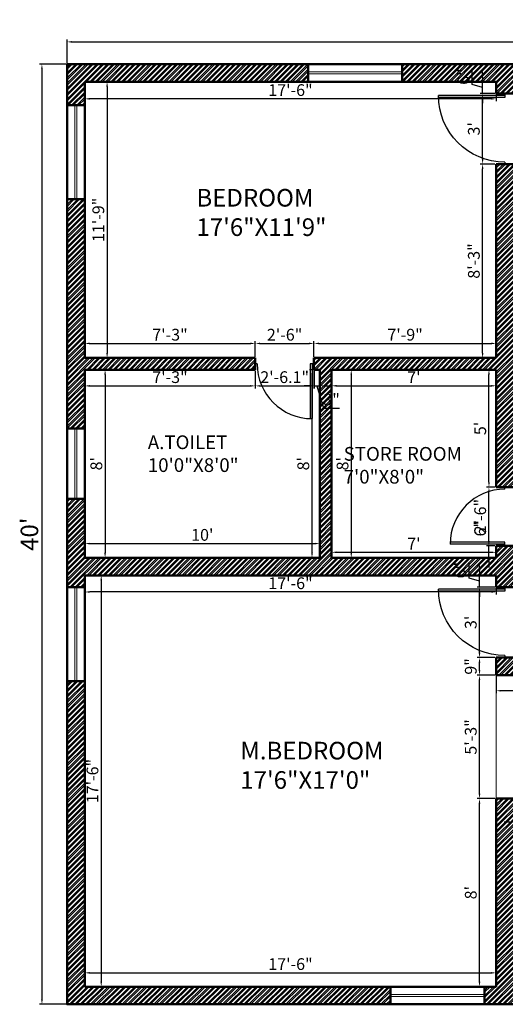
# Model space of a CAD drawing. Units: inches. Extents: x 3590 to 5167, y 65 to 1917.
# Tile 23 of 100: x 4396 to 4644, y 735 to 1238. Entities that reach past the tile are written whole.
import ezdxf

# ---------------------------------------------------------------- set-up
doc = ezdxf.new("R2010")
doc.units = ezdxf.units.IN
doc.linetypes.add('DASHED', pattern=[0.75, 0.5, -0.25])
for name, color, linetype, lineweight in [('A-ANNO-DIMS', 2, 'Continuous', 18), ('A-AREA-IDEN', 7, 'Continuous', 18), ('A-DOOR', 3, 'Continuous', 25), ('A-GLAZ', 4, 'Continuous', 18), ('A-WALL', 7, 'Continuous', 50), ('A-WALL-PATT', 251, 'Continuous', 13), ('S-BEAM-OVHD', 7, 'DASHED', 18)]:
    doc.layers.add(name, color=color, linetype=linetype, lineweight=lineweight)
doc.styles.get("Standard").update_dxf_attribs({"font": 'arial.ttf'})
doc.dimstyles.new('ISO-25', dxfattribs={"dimtxt": 9, "dimasz": 2.5, "dimexe": 1.25, "dimexo": 0.625, "dimtad": 1, "dimdec": 1, "dimlunit": 3, "dimtxsty": 'Standard', "dimcen": 2.5, "dimadec": 0, "dimazin": 0, "dimtfac": 1, "dimtdec": 1, "dimtmove": 0, "dimatfit": 3, "dimfxl": 1, "dimarcsym": 0})

# ---------------------------------------------------------------- blocks, each defined once
blk = doc.blocks.new('*D105')
at = {"layer": 'A-ANNO-DIMS', "color": 0, "lineweight": -2, "transparency": 16777216}
for p, q in [((4420.27, 1215.97), (4420.27, 1227.96)), ((4422.77, 1226.71), (5077.77, 1226.71)), ((5080.27, 1215.97), (5080.27, 1227.96))]:
    blk.add_line(p, q, dxfattribs=at)
at = {"layer": 'A-ANNO-DIMS', "color": 0, "transparency": 16777216}
for points in [[(4422.77, 1227.13), (4422.77, 1226.29), (4420.27, 1226.71)], [(5077.77, 1227.13), (5077.77, 1226.29), (5080.27, 1226.71)]]:
    blk.add_solid(points, dxfattribs=at)
at = {"layer": 'Defpoints', "color": 0, "transparency": 16777216}
for p in [(5080.27, 1226.71), (4420.27, 1215.35), (5080.27, 1215.35)]:
    blk.add_point(p, dxfattribs=at)
at = {"layer": 'A-ANNO-DIMS', "color": 0, "transparency": 16777216, "insert": (4750.27, 1231.91), "char_height": 9, "attachment_point": 5}
blk.add_mtext("55'", dxfattribs=at)
blk = doc.blocks.new('*D106')
at = {"layer": 'A-ANNO-DIMS', "color": 0, "lineweight": -2, "transparency": 16777216}
for p, q in [((4419.65, 1215.35), (4406.15, 1215.35)), ((4407.4, 1212.85), (4407.4, 737.85)), ((4419.65, 735.35), (4406.15, 735.35))]:
    blk.add_line(p, q, dxfattribs=at)
at = {"layer": 'A-ANNO-DIMS', "color": 0, "transparency": 16777216}
for points in [[(4406.98, 1212.85), (4407.82, 1212.85), (4407.4, 1215.35)], [(4406.98, 737.85), (4407.82, 737.85), (4407.4, 735.35)]]:
    blk.add_solid(points, dxfattribs=at)
at = {"layer": 'Defpoints', "color": 0, "transparency": 16777216}
for p in [(4420.27, 1215.35), (4407.4, 735.35), (4420.27, 735.35)]:
    blk.add_point(p, dxfattribs=at)
at = {"layer": 'A-ANNO-DIMS', "color": 0, "transparency": 16777216, "insert": (4402.18, 975.35), "char_height": 9, "attachment_point": 5, "rotation": 90}
blk.add_mtext("40'", dxfattribs=at)
blk = doc.blocks.new('D1')
for p, q in [((1, 0), (1, 34)), ((2, 0), (2, 33.99)), ((0, 0), (2, 0)), ((35, 0), (36, 0))]:
    blk.add_line(p, q)
at = {"ltscale": 0.5}
blk.add_arc((1, 0), 34, 0, 90, dxfattribs=at)
blk = doc.blocks.new('D2')
for p, q in [((1, 0), (1, 28)), ((2, 0), (2, 27.98)), ((0, 0), (2, 0)), ((29, 0), (30, 0))]:
    blk.add_line(p, q)
at = {"ltscale": 0.5}
blk.add_arc((1, 0), 28, 0, 90, dxfattribs=at)
blk = doc.blocks.new('*D107')
at = {"layer": 'A-ANNO-DIMS', "color": 0, "lineweight": -2, "transparency": 16777216}
for p, q in [((4429.27, 1205.72), (4429.27, 1196.39)), ((4639.27, 1205.72), (4639.27, 1196.39)), ((4636.77, 1197.64), (4431.77, 1197.64))]:
    blk.add_line(p, q, dxfattribs=at)
at = {"layer": 'A-ANNO-DIMS', "color": 0, "transparency": 16777216}
for points in [[(4431.77, 1198.06), (4431.77, 1197.22), (4429.27, 1197.64)], [(4636.77, 1198.06), (4636.77, 1197.22), (4639.27, 1197.64)]]:
    blk.add_solid(points, dxfattribs=at)
at = {"layer": 'Defpoints', "color": 0, "transparency": 16777216}
for p in [(4429.27, 1206.35), (4639.27, 1206.35), (4429.27, 1197.64)]:
    blk.add_point(p, dxfattribs=at)
at = {"layer": 'A-ANNO-DIMS', "color": 0, "transparency": 16777216, "insert": (4534.27, 1201.33), "char_height": 6, "attachment_point": 5}
blk.add_mtext('17\'-6"', dxfattribs=at)
blk = doc.blocks.new('*D108')
at = {"layer": 'A-ANNO-DIMS', "color": 0, "lineweight": -2, "transparency": 16777216}
for p, q in [((4429.9, 1206.35), (4441.91, 1206.35)), ((4440.66, 1203.85), (4440.66, 1067.85)), ((4429.9, 1065.35), (4441.91, 1065.35))]:
    blk.add_line(p, q, dxfattribs=at)
at = {"layer": 'A-ANNO-DIMS', "color": 0, "transparency": 16777216}
for points in [[(4440.24, 1203.85), (4441.08, 1203.85), (4440.66, 1206.35)], [(4440.24, 1067.85), (4441.08, 1067.85), (4440.66, 1065.35)]]:
    blk.add_solid(points, dxfattribs=at)
at = {"layer": 'Defpoints', "color": 0, "transparency": 16777216}
for p in [(4429.27, 1206.35), (4429.27, 1065.35), (4440.66, 1065.35)]:
    blk.add_point(p, dxfattribs=at)
at = {"layer": 'A-ANNO-DIMS', "color": 0, "transparency": 16777216, "insert": (4436.97, 1135.85), "char_height": 6, "attachment_point": 5, "rotation": 90}
blk.add_mtext('11\'-9"', dxfattribs=at)
blk = doc.blocks.new('*D109')
at = {"layer": 'A-ANNO-DIMS', "color": 0, "lineweight": -2, "transparency": 16777216}
for p, q in [((4429.27, 1065.97), (4429.27, 1074)), ((4431.77, 1072.75), (4513.77, 1072.75)), ((4516.27, 1065.97), (4516.27, 1074))]:
    blk.add_line(p, q, dxfattribs=at)
at = {"layer": 'A-ANNO-DIMS', "color": 0, "transparency": 16777216}
for points in [[(4431.77, 1073.17), (4431.77, 1072.33), (4429.27, 1072.75)], [(4513.77, 1073.17), (4513.77, 1072.33), (4516.27, 1072.75)]]:
    blk.add_solid(points, dxfattribs=at)
at = {"layer": 'Defpoints', "color": 0, "transparency": 16777216}
for p in [(4516.27, 1072.75), (4429.27, 1065.35), (4516.27, 1065.35)]:
    blk.add_point(p, dxfattribs=at)
at = {"layer": 'A-ANNO-DIMS', "color": 0, "transparency": 16777216, "insert": (4472.77, 1076.44), "char_height": 6, "attachment_point": 5}
blk.add_mtext('7\'-3"', dxfattribs=at)
blk = doc.blocks.new('*D110')
at = {"layer": 'A-ANNO-DIMS', "color": 0, "lineweight": -2, "transparency": 16777216}
for p, q in [((4516.27, 1065.97), (4516.27, 1074)), ((4518.77, 1072.75), (4543.77, 1072.75)), ((4546.27, 1065.97), (4546.27, 1074))]:
    blk.add_line(p, q, dxfattribs=at)
at = {"layer": 'A-ANNO-DIMS', "color": 0, "transparency": 16777216}
for points in [[(4518.77, 1073.17), (4518.77, 1072.33), (4516.27, 1072.75)], [(4543.77, 1073.17), (4543.77, 1072.33), (4546.27, 1072.75)]]:
    blk.add_solid(points, dxfattribs=at)
at = {"layer": 'Defpoints', "color": 0, "transparency": 16777216}
for p in [(4546.27, 1072.75), (4516.27, 1065.35), (4546.27, 1065.35)]:
    blk.add_point(p, dxfattribs=at)
at = {"layer": 'A-ANNO-DIMS', "color": 0, "transparency": 16777216, "insert": (4531.27, 1076.44), "char_height": 6, "attachment_point": 5}
blk.add_mtext('2\'-6"', dxfattribs=at)
blk = doc.blocks.new('*D111')
at = {"layer": 'A-ANNO-DIMS', "color": 0, "lineweight": -2, "transparency": 16777216}
for p, q in [((4546.27, 1065.97), (4546.27, 1074)), ((4548.77, 1072.75), (4636.77, 1072.75)), ((4639.27, 1065.97), (4639.27, 1074))]:
    blk.add_line(p, q, dxfattribs=at)
at = {"layer": 'A-ANNO-DIMS', "color": 0, "transparency": 16777216}
for points in [[(4548.77, 1073.17), (4548.77, 1072.33), (4546.27, 1072.75)], [(4636.77, 1073.17), (4636.77, 1072.33), (4639.27, 1072.75)]]:
    blk.add_solid(points, dxfattribs=at)
at = {"layer": 'Defpoints', "color": 0, "transparency": 16777216}
for p in [(4639.27, 1072.75), (4546.27, 1065.35), (4639.27, 1065.35)]:
    blk.add_point(p, dxfattribs=at)
at = {"layer": 'A-ANNO-DIMS', "color": 0, "transparency": 16777216, "insert": (4592.77, 1076.44), "char_height": 6, "attachment_point": 5}
blk.add_mtext('7\'-9"', dxfattribs=at)
blk = doc.blocks.new('*D112')
at = {"layer": 'A-ANNO-DIMS', "color": 0, "lineweight": -2, "transparency": 16777216}
for p, q in [((4638.65, 1164.35), (4631.09, 1164.35)), ((4632.34, 1067.85), (4632.34, 1161.85)), ((4638.65, 1065.35), (4631.09, 1065.35))]:
    blk.add_line(p, q, dxfattribs=at)
at = {"layer": 'A-ANNO-DIMS', "color": 0, "transparency": 16777216}
for points in [[(4631.93, 1161.85), (4632.76, 1161.85), (4632.34, 1164.35)], [(4631.93, 1067.85), (4632.76, 1067.85), (4632.34, 1065.35)]]:
    blk.add_solid(points, dxfattribs=at)
at = {"layer": 'Defpoints', "color": 0, "transparency": 16777216}
for p in [(4632.34, 1164.35), (4639.27, 1164.35), (4639.27, 1065.35)]:
    blk.add_point(p, dxfattribs=at)
at = {"layer": 'A-ANNO-DIMS', "color": 0, "transparency": 16777216, "insert": (4628.65, 1114.85), "char_height": 6, "attachment_point": 5, "rotation": 90}
blk.add_mtext('8\'-3"', dxfattribs=at)
blk = doc.blocks.new('*D113')
at = {"layer": 'A-ANNO-DIMS', "color": 0, "lineweight": -2, "transparency": 16777216}
for p, q in [((4638.65, 1200.35), (4631.09, 1200.35)), ((4632.34, 1166.85), (4632.34, 1197.85)), ((4638.65, 1164.35), (4631.09, 1164.35))]:
    blk.add_line(p, q, dxfattribs=at)
at = {"layer": 'A-ANNO-DIMS', "color": 0, "transparency": 16777216}
for points in [[(4631.93, 1197.85), (4632.76, 1197.85), (4632.34, 1200.35)], [(4631.93, 1166.85), (4632.76, 1166.85), (4632.34, 1164.35)]]:
    blk.add_solid(points, dxfattribs=at)
at = {"layer": 'Defpoints', "color": 0, "transparency": 16777216}
for p in [(4632.34, 1200.35), (4639.27, 1200.35), (4639.27, 1164.35)]:
    blk.add_point(p, dxfattribs=at)
at = {"layer": 'A-ANNO-DIMS', "color": 0, "transparency": 16777216, "insert": (4628.65, 1182.35), "char_height": 6, "attachment_point": 5, "rotation": 90}
blk.add_mtext("3'", dxfattribs=at)
blk = doc.blocks.new('*D114')
at = {"layer": 'A-ANNO-DIMS', "color": 0, "lineweight": -2, "transparency": 16777216}
for p, q in [((4627.09, 1204.92), (4627.09, 1213.1)), ((4632.34, 1208.85), (4632.34, 1211.35)), ((4632.34, 1203.35), (4627.09, 1204.92)), ((4638.65, 1206.35), (4631.09, 1206.35)), ((4632.34, 1200.35), (4632.34, 1206.35)), ((4632.34, 1200.35), (4632.34, 1206.35)), ((4638.65, 1200.35), (4631.09, 1200.35)), ((4632.34, 1197.85), (4632.34, 1195.35))]:
    blk.add_line(p, q, dxfattribs=at)
at = {"layer": 'A-ANNO-DIMS', "color": 0, "transparency": 16777216}
for points in [[(4631.93, 1208.85), (4632.76, 1208.85), (4632.34, 1206.35)], [(4631.93, 1197.85), (4632.76, 1197.85), (4632.34, 1200.35)]]:
    blk.add_solid(points, dxfattribs=at)
at = {"layer": 'Defpoints', "color": 0, "transparency": 16777216}
for p in [(4632.34, 1206.35), (4639.27, 1206.35), (4639.27, 1200.35)]:
    blk.add_point(p, dxfattribs=at)
at = {"layer": 'A-ANNO-DIMS', "color": 0, "transparency": 16777216, "insert": (4623.4, 1209.01), "char_height": 6, "attachment_point": 5, "rotation": 90}
blk.add_mtext('6"', dxfattribs=at)
blk = doc.blocks.new('*D115')
at = {"layer": 'A-ANNO-DIMS', "color": 0, "lineweight": -2, "transparency": 16777216}
for p, q in [((4429.9, 1059.35), (4440.89, 1059.35)), ((4439.64, 1056.85), (4439.64, 965.85)), ((4429.9, 963.35), (4440.89, 963.35))]:
    blk.add_line(p, q, dxfattribs=at)
at = {"layer": 'A-ANNO-DIMS', "color": 0, "transparency": 16777216}
for points in [[(4439.22, 1056.85), (4440.05, 1056.85), (4439.64, 1059.35)], [(4439.22, 965.85), (4440.05, 965.85), (4439.64, 963.35)]]:
    blk.add_solid(points, dxfattribs=at)
at = {"layer": 'Defpoints', "color": 0, "transparency": 16777216}
for p in [(4429.27, 1059.35), (4429.27, 963.35), (4439.64, 963.35)]:
    blk.add_point(p, dxfattribs=at)
at = {"layer": 'A-ANNO-DIMS', "color": 0, "transparency": 16777216, "insert": (4435.95, 1011.35), "char_height": 6, "attachment_point": 5, "rotation": 90}
blk.add_mtext("8'", dxfattribs=at)
blk = doc.blocks.new('*D116')
at = {"layer": 'A-ANNO-DIMS', "color": 0, "lineweight": -2, "transparency": 16777216}
for p, q in [((4429.27, 963.97), (4429.27, 971.82)), ((4431.77, 970.57), (4546.77, 970.57)), ((4549.27, 963.97), (4549.27, 971.82))]:
    blk.add_line(p, q, dxfattribs=at)
at = {"layer": 'A-ANNO-DIMS', "color": 0, "transparency": 16777216}
for points in [[(4431.77, 970.98), (4431.77, 970.15), (4429.27, 970.57)], [(4546.77, 970.98), (4546.77, 970.15), (4549.27, 970.57)]]:
    blk.add_solid(points, dxfattribs=at)
at = {"layer": 'Defpoints', "color": 0, "transparency": 16777216}
for p in [(4549.27, 970.57), (4429.27, 963.35), (4549.27, 963.35)]:
    blk.add_point(p, dxfattribs=at)
at = {"layer": 'A-ANNO-DIMS', "color": 0, "transparency": 16777216, "insert": (4489.27, 974.25), "char_height": 6, "attachment_point": 5}
blk.add_mtext("10'", dxfattribs=at)
blk = doc.blocks.new('*D117')
at = {"layer": 'A-ANNO-DIMS', "color": 0, "lineweight": -2, "transparency": 16777216}
for p, q in [((4548.65, 1059.35), (4544.02, 1059.35)), ((4545.27, 965.85), (4545.27, 1056.85)), ((4548.65, 963.35), (4544.02, 963.35))]:
    blk.add_line(p, q, dxfattribs=at)
at = {"layer": 'A-ANNO-DIMS', "color": 0, "transparency": 16777216}
for points in [[(4544.86, 1056.85), (4545.69, 1056.85), (4545.27, 1059.35)], [(4544.86, 965.85), (4545.69, 965.85), (4545.27, 963.35)]]:
    blk.add_solid(points, dxfattribs=at)
at = {"layer": 'Defpoints', "color": 0, "transparency": 16777216}
for p in [(4545.27, 1059.35), (4549.27, 1059.35), (4549.27, 963.35)]:
    blk.add_point(p, dxfattribs=at)
at = {"layer": 'A-ANNO-DIMS', "color": 0, "transparency": 16777216, "insert": (4541.59, 1011.35), "char_height": 6, "attachment_point": 5, "rotation": 90}
blk.add_mtext("8'", dxfattribs=at)
blk = doc.blocks.new('*D118')
at = {"layer": 'A-ANNO-DIMS', "color": 0, "lineweight": -2, "transparency": 16777216}
for p, q in [((4429.27, 1058.72), (4429.27, 1049.83)), ((4516.27, 1058.72), (4516.27, 1049.83)), ((4431.77, 1051.08), (4513.77, 1051.08))]:
    blk.add_line(p, q, dxfattribs=at)
at = {"layer": 'A-ANNO-DIMS', "color": 0, "transparency": 16777216}
for points in [[(4431.77, 1051.5), (4431.77, 1050.67), (4429.27, 1051.08)], [(4513.77, 1051.5), (4513.77, 1050.67), (4516.27, 1051.08)]]:
    blk.add_solid(points, dxfattribs=at)
at = {"layer": 'Defpoints', "color": 0, "transparency": 16777216}
for p in [(4429.27, 1059.35), (4516.27, 1059.35), (4516.27, 1051.08)]:
    blk.add_point(p, dxfattribs=at)
at = {"layer": 'A-ANNO-DIMS', "color": 0, "transparency": 16777216, "insert": (4472.77, 1054.77), "char_height": 6, "attachment_point": 5}
blk.add_mtext('7\'-3"', dxfattribs=at)
blk = doc.blocks.new('*D119')
at = {"layer": 'A-ANNO-DIMS', "color": 0, "lineweight": -2, "transparency": 16777216}
for p, q in [((4516.27, 1058.72), (4516.27, 1049.83)), ((4546.34, 1058.72), (4546.34, 1049.83)), ((4518.77, 1051.08), (4543.84, 1051.08))]:
    blk.add_line(p, q, dxfattribs=at)
at = {"layer": 'A-ANNO-DIMS', "color": 0, "transparency": 16777216}
for points in [[(4518.77, 1051.5), (4518.77, 1050.67), (4516.27, 1051.08)], [(4543.84, 1051.5), (4543.84, 1050.67), (4546.34, 1051.08)]]:
    blk.add_solid(points, dxfattribs=at)
at = {"layer": 'Defpoints', "color": 0, "transparency": 16777216}
for p in [(4516.27, 1059.35), (4546.34, 1059.35), (4546.34, 1051.08)]:
    blk.add_point(p, dxfattribs=at)
at = {"layer": 'A-ANNO-DIMS', "color": 0, "transparency": 16777216, "insert": (4531.31, 1054.77), "char_height": 6, "attachment_point": 5}
blk.add_mtext('2\'-6.1"', dxfattribs=at)
blk = doc.blocks.new('*D120')
at = {"layer": 'A-ANNO-DIMS', "color": 0, "lineweight": -2, "transparency": 16777216}
for p, q in [((4546.27, 1058.72), (4546.27, 1049.83)), ((4549.27, 1058.72), (4549.27, 1049.83)), ((4543.77, 1051.08), (4541.27, 1051.08)), ((4546.27, 1051.08), (4549.27, 1051.08)), ((4546.27, 1051.08), (4549.27, 1051.08)), ((4547.77, 1051.08), (4551.19, 1039.7)), ((4551.77, 1051.08), (4554.27, 1051.08)), ((4551.19, 1039.7), (4559.33, 1039.7))]:
    blk.add_line(p, q, dxfattribs=at)
at = {"layer": 'A-ANNO-DIMS', "color": 0, "transparency": 16777216}
for points in [[(4543.77, 1051.5), (4543.77, 1050.67), (4546.27, 1051.08)], [(4551.77, 1051.5), (4551.77, 1050.67), (4549.27, 1051.08)]]:
    blk.add_solid(points, dxfattribs=at)
at = {"layer": 'Defpoints', "color": 0, "transparency": 16777216}
for p in [(4546.27, 1059.35), (4549.27, 1059.35), (4549.27, 1051.08)]:
    blk.add_point(p, dxfattribs=at)
at = {"layer": 'A-ANNO-DIMS', "color": 0, "transparency": 16777216, "insert": (4555.26, 1043.39), "char_height": 6, "attachment_point": 5}
blk.add_mtext('3"', dxfattribs=at)
blk = doc.blocks.new('*D121')
at = {"layer": 'A-ANNO-DIMS', "color": 0, "lineweight": -2, "transparency": 16777216}
for p, q in [((4555.27, 1058.72), (4555.27, 1049.87)), ((4639.27, 1058.72), (4639.27, 1049.87)), ((4557.77, 1051.12), (4636.77, 1051.12))]:
    blk.add_line(p, q, dxfattribs=at)
at = {"layer": 'A-ANNO-DIMS', "color": 0, "transparency": 16777216}
for points in [[(4557.77, 1051.54), (4557.77, 1050.71), (4555.27, 1051.12)], [(4636.77, 1051.54), (4636.77, 1050.71), (4639.27, 1051.12)]]:
    blk.add_solid(points, dxfattribs=at)
at = {"layer": 'Defpoints', "color": 0, "transparency": 16777216}
for p in [(4555.27, 1059.35), (4639.27, 1059.35), (4639.27, 1051.12)]:
    blk.add_point(p, dxfattribs=at)
at = {"layer": 'A-ANNO-DIMS', "color": 0, "transparency": 16777216, "insert": (4597.27, 1054.75), "char_height": 6, "attachment_point": 5}
blk.add_mtext("7'", dxfattribs=at)
blk = doc.blocks.new('*D122')
at = {"layer": 'A-ANNO-DIMS', "color": 0, "lineweight": -2, "transparency": 16777216}
for p, q in [((4555.9, 1059.35), (4566.54, 1059.35)), ((4565.29, 1056.85), (4565.29, 965.85)), ((4555.9, 963.35), (4566.54, 963.35))]:
    blk.add_line(p, q, dxfattribs=at)
at = {"layer": 'A-ANNO-DIMS', "color": 0, "transparency": 16777216}
for points in [[(4564.88, 1056.85), (4565.71, 1056.85), (4565.29, 1059.35)], [(4564.88, 965.85), (4565.71, 965.85), (4565.29, 963.35)]]:
    blk.add_solid(points, dxfattribs=at)
at = {"layer": 'Defpoints', "color": 0, "transparency": 16777216}
for p in [(4555.27, 1059.35), (4555.27, 963.35), (4565.29, 963.35)]:
    blk.add_point(p, dxfattribs=at)
at = {"layer": 'A-ANNO-DIMS', "color": 0, "transparency": 16777216, "insert": (4561.61, 1011.35), "char_height": 6, "attachment_point": 5, "rotation": 90}
blk.add_mtext("8'", dxfattribs=at)
blk = doc.blocks.new('*D123')
at = {"layer": 'A-ANNO-DIMS', "color": 0, "lineweight": -2, "transparency": 16777216}
for p, q in [((4555.27, 963.97), (4555.27, 967.37)), ((4557.77, 966.12), (4636.77, 966.12)), ((4639.27, 963.97), (4639.27, 967.37))]:
    blk.add_line(p, q, dxfattribs=at)
at = {"layer": 'A-ANNO-DIMS', "color": 0, "transparency": 16777216}
for points in [[(4557.77, 966.54), (4557.77, 965.71), (4555.27, 966.12)], [(4636.77, 966.54), (4636.77, 965.71), (4639.27, 966.12)]]:
    blk.add_solid(points, dxfattribs=at)
at = {"layer": 'Defpoints', "color": 0, "transparency": 16777216}
for p in [(4639.27, 966.12), (4555.27, 963.35), (4639.27, 963.35)]:
    blk.add_point(p, dxfattribs=at)
at = {"layer": 'A-ANNO-DIMS', "color": 0, "transparency": 16777216, "insert": (4597.27, 969.75), "char_height": 6, "attachment_point": 5}
blk.add_mtext("7'", dxfattribs=at)
blk = doc.blocks.new('*D124')
at = {"layer": 'A-ANNO-DIMS', "color": 0, "lineweight": -2, "transparency": 16777216}
for p, q in [((4635.58, 971.85), (4635.58, 982.52)), ((4638.65, 969.35), (4634.33, 969.35)), ((4635.58, 963.35), (4635.58, 969.35)), ((4638.65, 963.35), (4634.33, 963.35)), ((4635.58, 960.85), (4635.58, 958.35))]:
    blk.add_line(p, q, dxfattribs=at)
at = {"layer": 'A-ANNO-DIMS', "color": 0, "transparency": 16777216}
for points in [[(4635.17, 971.85), (4636, 971.85), (4635.58, 969.35)], [(4635.17, 960.85), (4636, 960.85), (4635.58, 963.35)]]:
    blk.add_solid(points, dxfattribs=at)
at = {"layer": 'Defpoints', "color": 0, "transparency": 16777216}
for p in [(4635.58, 969.35), (4639.27, 969.35), (4639.27, 963.35)]:
    blk.add_point(p, dxfattribs=at)
at = {"layer": 'A-ANNO-DIMS', "color": 0, "transparency": 16777216, "insert": (4631.89, 978.43), "char_height": 6, "attachment_point": 5, "rotation": 90}
blk.add_mtext('6"', dxfattribs=at)
blk = doc.blocks.new('*D125')
at = {"layer": 'A-ANNO-DIMS', "color": 0, "lineweight": -2, "transparency": 16777216}
for p, q in [((4638.65, 999.35), (4634.33, 999.35)), ((4635.58, 971.85), (4635.58, 996.85)), ((4638.65, 969.35), (4634.33, 969.35))]:
    blk.add_line(p, q, dxfattribs=at)
at = {"layer": 'A-ANNO-DIMS', "color": 0, "transparency": 16777216}
for points in [[(4635.17, 996.85), (4636, 996.85), (4635.58, 999.35)], [(4635.17, 971.85), (4636, 971.85), (4635.58, 969.35)]]:
    blk.add_solid(points, dxfattribs=at)
at = {"layer": 'Defpoints', "color": 0, "transparency": 16777216}
for p in [(4635.58, 999.35), (4639.27, 999.35), (4639.27, 969.35)]:
    blk.add_point(p, dxfattribs=at)
at = {"layer": 'A-ANNO-DIMS', "color": 0, "transparency": 16777216, "insert": (4631.89, 984.35), "char_height": 6, "attachment_point": 5, "rotation": 90}
blk.add_mtext('2\'-6"', dxfattribs=at)
blk = doc.blocks.new('*D126')
at = {"layer": 'A-ANNO-DIMS', "color": 0, "lineweight": -2, "transparency": 16777216}
for p, q in [((4638.65, 1059.35), (4634.33, 1059.35)), ((4635.58, 1001.85), (4635.58, 1056.85)), ((4638.65, 999.35), (4634.33, 999.35))]:
    blk.add_line(p, q, dxfattribs=at)
at = {"layer": 'A-ANNO-DIMS', "color": 0, "transparency": 16777216}
for points in [[(4635.17, 1056.85), (4636, 1056.85), (4635.58, 1059.35)], [(4635.17, 1001.85), (4636, 1001.85), (4635.58, 999.35)]]:
    blk.add_solid(points, dxfattribs=at)
at = {"layer": 'Defpoints', "color": 0, "transparency": 16777216}
for p in [(4635.58, 1059.35), (4639.27, 1059.35), (4639.27, 999.35)]:
    blk.add_point(p, dxfattribs=at)
at = {"layer": 'A-ANNO-DIMS', "color": 0, "transparency": 16777216, "insert": (4631.91, 1029.35), "char_height": 6, "attachment_point": 5, "rotation": 90}
blk.add_mtext("5'", dxfattribs=at)
blk = doc.blocks.new('*D127')
at = {"layer": 'A-ANNO-DIMS', "color": 0, "lineweight": -2, "transparency": 16777216}
for p, q in [((4429.27, 953.72), (4429.27, 944.61)), ((4639.27, 953.72), (4639.27, 944.61)), ((4636.77, 945.86), (4431.77, 945.86))]:
    blk.add_line(p, q, dxfattribs=at)
at = {"layer": 'A-ANNO-DIMS', "color": 0, "transparency": 16777216}
for points in [[(4431.77, 946.28), (4431.77, 945.44), (4429.27, 945.86)], [(4636.77, 946.28), (4636.77, 945.44), (4639.27, 945.86)]]:
    blk.add_solid(points, dxfattribs=at)
at = {"layer": 'Defpoints', "color": 0, "transparency": 16777216}
for p in [(4429.27, 954.35), (4639.27, 954.35), (4429.27, 945.86)]:
    blk.add_point(p, dxfattribs=at)
at = {"layer": 'A-ANNO-DIMS', "color": 0, "transparency": 16777216, "insert": (4534.27, 949.55), "char_height": 6, "attachment_point": 5}
blk.add_mtext('17\'-6"', dxfattribs=at)
blk = doc.blocks.new('*D128')
at = {"layer": 'A-ANNO-DIMS', "color": 0, "lineweight": -2, "transparency": 16777216}
for p, q in [((4429.9, 954.35), (4438.92, 954.35)), ((4437.67, 951.85), (4437.67, 746.85)), ((4429.9, 744.35), (4438.92, 744.35))]:
    blk.add_line(p, q, dxfattribs=at)
at = {"layer": 'A-ANNO-DIMS', "color": 0, "transparency": 16777216}
for points in [[(4437.25, 951.85), (4438.08, 951.85), (4437.67, 954.35)], [(4437.25, 746.85), (4438.08, 746.85), (4437.67, 744.35)]]:
    blk.add_solid(points, dxfattribs=at)
at = {"layer": 'Defpoints', "color": 0, "transparency": 16777216}
for p in [(4429.27, 954.35), (4429.27, 744.35), (4437.67, 744.35)]:
    blk.add_point(p, dxfattribs=at)
at = {"layer": 'A-ANNO-DIMS', "color": 0, "transparency": 16777216, "insert": (4433.98, 849.35), "char_height": 6, "attachment_point": 5, "rotation": 90}
blk.add_mtext('17\'-6"', dxfattribs=at)
blk = doc.blocks.new('*D129')
at = {"layer": 'A-ANNO-DIMS', "color": 0, "lineweight": -2, "transparency": 16777216}
for p, q in [((4429.27, 744.97), (4429.27, 752.66)), ((4431.77, 751.41), (4636.77, 751.41)), ((4639.27, 744.97), (4639.27, 752.66))]:
    blk.add_line(p, q, dxfattribs=at)
at = {"layer": 'A-ANNO-DIMS', "color": 0, "transparency": 16777216}
for points in [[(4431.77, 751.83), (4431.77, 751), (4429.27, 751.41)], [(4636.77, 751.83), (4636.77, 751), (4639.27, 751.41)]]:
    blk.add_solid(points, dxfattribs=at)
at = {"layer": 'Defpoints', "color": 0, "transparency": 16777216}
for p in [(4639.27, 751.41), (4429.27, 744.35), (4639.27, 744.35)]:
    blk.add_point(p, dxfattribs=at)
at = {"layer": 'A-ANNO-DIMS', "color": 0, "transparency": 16777216, "insert": (4534.27, 755.1), "char_height": 6, "attachment_point": 5}
blk.add_mtext('17\'-6"', dxfattribs=at)
blk = doc.blocks.new('*D130')
at = {"layer": 'A-ANNO-DIMS', "color": 0, "lineweight": -2, "transparency": 16777216}
for p, q in [((4638.65, 840.35), (4629.51, 840.35)), ((4630.76, 746.85), (4630.76, 837.85)), ((4638.65, 744.35), (4629.51, 744.35))]:
    blk.add_line(p, q, dxfattribs=at)
at = {"layer": 'A-ANNO-DIMS', "color": 0, "transparency": 16777216}
for points in [[(4630.35, 837.85), (4631.18, 837.85), (4630.76, 840.35)], [(4630.35, 746.85), (4631.18, 746.85), (4630.76, 744.35)]]:
    blk.add_solid(points, dxfattribs=at)
at = {"layer": 'Defpoints', "color": 0, "transparency": 16777216}
for p in [(4630.76, 840.35), (4639.27, 840.35), (4639.27, 744.35)]:
    blk.add_point(p, dxfattribs=at)
at = {"layer": 'A-ANNO-DIMS', "color": 0, "transparency": 16777216, "insert": (4627.08, 792.35), "char_height": 6, "attachment_point": 5, "rotation": 90}
blk.add_mtext("8'", dxfattribs=at)
blk = doc.blocks.new('*D131')
at = {"layer": 'A-ANNO-DIMS', "color": 0, "lineweight": -2, "transparency": 16777216}
for p, q in [((4638.65, 903.35), (4629.51, 903.35)), ((4630.76, 842.85), (4630.76, 900.85)), ((4638.65, 840.35), (4629.51, 840.35))]:
    blk.add_line(p, q, dxfattribs=at)
at = {"layer": 'A-ANNO-DIMS', "color": 0, "transparency": 16777216}
for points in [[(4630.35, 900.85), (4631.18, 900.85), (4630.76, 903.35)], [(4630.35, 842.85), (4631.18, 842.85), (4630.76, 840.35)]]:
    blk.add_solid(points, dxfattribs=at)
at = {"layer": 'Defpoints', "color": 0, "transparency": 16777216}
for p in [(4630.76, 903.35), (4639.27, 903.35), (4639.27, 840.35)]:
    blk.add_point(p, dxfattribs=at)
at = {"layer": 'A-ANNO-DIMS', "color": 0, "transparency": 16777216, "insert": (4627.07, 871.85), "char_height": 6, "attachment_point": 5, "rotation": 90}
blk.add_mtext('5\'-3"', dxfattribs=at)
blk = doc.blocks.new('*D132')
at = {"layer": 'A-ANNO-DIMS', "color": 0, "lineweight": -2, "transparency": 16777216}
for p, q in [((4638.65, 912.35), (4629.51, 912.35)), ((4630.76, 905.85), (4630.76, 909.85)), ((4638.65, 903.35), (4629.51, 903.35))]:
    blk.add_line(p, q, dxfattribs=at)
at = {"layer": 'A-ANNO-DIMS', "color": 0, "transparency": 16777216}
for points in [[(4630.35, 909.85), (4631.18, 909.85), (4630.76, 912.35)], [(4630.35, 905.85), (4631.18, 905.85), (4630.76, 903.35)]]:
    blk.add_solid(points, dxfattribs=at)
at = {"layer": 'Defpoints', "color": 0, "transparency": 16777216}
for p in [(4630.76, 912.35), (4639.27, 912.35), (4639.27, 903.35)]:
    blk.add_point(p, dxfattribs=at)
at = {"layer": 'A-ANNO-DIMS', "color": 0, "transparency": 16777216, "insert": (4627.08, 907.85), "char_height": 6, "attachment_point": 5, "rotation": 90}
blk.add_mtext('9"', dxfattribs=at)
blk = doc.blocks.new('*D133')
at = {"layer": 'A-ANNO-DIMS', "color": 0, "lineweight": -2, "transparency": 16777216}
for p, q in [((4638.65, 948.35), (4629.51, 948.35)), ((4630.76, 914.85), (4630.76, 945.85)), ((4638.65, 912.35), (4629.51, 912.35))]:
    blk.add_line(p, q, dxfattribs=at)
at = {"layer": 'A-ANNO-DIMS', "color": 0, "transparency": 16777216}
for points in [[(4630.35, 945.85), (4631.18, 945.85), (4630.76, 948.35)], [(4630.35, 914.85), (4631.18, 914.85), (4630.76, 912.35)]]:
    blk.add_solid(points, dxfattribs=at)
at = {"layer": 'Defpoints', "color": 0, "transparency": 16777216}
for p in [(4630.76, 948.35), (4639.27, 948.35), (4639.27, 912.35)]:
    blk.add_point(p, dxfattribs=at)
at = {"layer": 'A-ANNO-DIMS', "color": 0, "transparency": 16777216, "insert": (4627.07, 930.35), "char_height": 6, "attachment_point": 5, "rotation": 90}
blk.add_mtext("3'", dxfattribs=at)
blk = doc.blocks.new('*D134')
at = {"layer": 'A-ANNO-DIMS', "color": 0, "lineweight": -2, "transparency": 16777216}
for p, q in [((4625.51, 952.92), (4625.51, 961.1)), ((4630.76, 956.85), (4630.76, 959.35)), ((4630.76, 951.35), (4625.51, 952.92)), ((4638.65, 954.35), (4629.51, 954.35)), ((4630.76, 948.35), (4630.76, 954.35)), ((4630.76, 948.35), (4630.76, 954.35)), ((4638.65, 948.35), (4629.51, 948.35)), ((4630.76, 945.85), (4630.76, 943.35))]:
    blk.add_line(p, q, dxfattribs=at)
at = {"layer": 'A-ANNO-DIMS', "color": 0, "transparency": 16777216}
for points in [[(4630.35, 956.85), (4631.18, 956.85), (4630.76, 954.35)], [(4630.35, 945.85), (4631.18, 945.85), (4630.76, 948.35)]]:
    blk.add_solid(points, dxfattribs=at)
at = {"layer": 'Defpoints', "color": 0, "transparency": 16777216}
for p in [(4630.76, 954.35), (4639.27, 954.35), (4639.27, 948.35)]:
    blk.add_point(p, dxfattribs=at)
at = {"layer": 'A-ANNO-DIMS', "color": 0, "transparency": 16777216, "insert": (4621.82, 957.01), "char_height": 6, "attachment_point": 5, "rotation": 90}
blk.add_mtext('6"', dxfattribs=at)
blk = doc.blocks.new('*D135')
at = {"layer": 'A-ANNO-DIMS', "color": 0, "lineweight": -2, "transparency": 16777216}
for p, q in [((4639.27, 902.72), (4639.27, 894.19)), ((4687.27, 902.72), (4687.27, 894.19)), ((4684.77, 895.44), (4641.77, 895.44))]:
    blk.add_line(p, q, dxfattribs=at)
at = {"layer": 'A-ANNO-DIMS', "color": 0, "transparency": 16777216}
for points in [[(4641.77, 895.86), (4641.77, 895.03), (4639.27, 895.44)], [(4684.77, 895.86), (4684.77, 895.03), (4687.27, 895.44)]]:
    blk.add_solid(points, dxfattribs=at)
at = {"layer": 'Defpoints', "color": 0, "transparency": 16777216}
for p in [(4639.27, 903.35), (4687.27, 903.35), (4639.27, 895.44)]:
    blk.add_point(p, dxfattribs=at)
at = {"layer": 'A-ANNO-DIMS', "color": 0, "transparency": 16777216, "insert": (4663.27, 899.07), "char_height": 6, "attachment_point": 5}
blk.add_mtext("4'", dxfattribs=at)
blk = doc.blocks.new('*D137')
at = {"layer": 'A-ANNO-DIMS', "color": 0, "lineweight": -2, "transparency": 16777216}
for p, q in [((4648.27, 830.72), (4648.27, 827.11)), ((4651.27, 830.72), (4651.27, 827.11)), ((4645.77, 828.36), (4643.27, 828.36)), ((4648.27, 828.36), (4651.27, 828.36)), ((4653.77, 828.36), (4664.42, 828.36))]:
    blk.add_line(p, q, dxfattribs=at)
at = {"layer": 'A-ANNO-DIMS', "color": 0, "transparency": 16777216}
for points in [[(4645.77, 828.78), (4645.77, 827.94), (4648.27, 828.36)], [(4653.77, 828.78), (4653.77, 827.94), (4651.27, 828.36)]]:
    blk.add_solid(points, dxfattribs=at)
at = {"layer": 'Defpoints', "color": 0, "transparency": 16777216}
for p in [(4648.27, 831.35), (4651.27, 831.35), (4651.27, 828.36)]:
    blk.add_point(p, dxfattribs=at)
at = {"layer": 'A-ANNO-DIMS', "color": 0, "transparency": 16777216, "insert": (4660.35, 832.05), "char_height": 6, "attachment_point": 5}
blk.add_mtext('3"', dxfattribs=at)

msp = doc.modelspace()

# ---------------------------------------------------------------- hatches: boundary and pattern name
at = {"layer": 'A-WALL-PATT', "transparency": 33554687}
h = msp.add_hatch(dxfattribs=at)
h.set_pattern_fill('ANSI32', color=256, scale=0.2)
h.set_pattern_definition([(45, (0, -590.6538), (-1.3470384, 1.3470384), []), (45, (0.898, -590.6538), (-1.3470384, 1.3470384), [])])
h.paths.add_polyline_path([(4684.27, 1215.35), (4591.27, 1215.35), (4591.27, 1206.35), (4639.27, 1206.35), (4639.27, 1200.35), (4648.27, 1200.35), (4648.27, 1206.35), (4684.27, 1206.35)])
h.paths.add_polyline_path([(4543.27, 1215.35), (4420.27, 1215.35), (4420.27, 1194.35), (4429.27, 1194.35), (4429.27, 1206.35), (4445.92, 1206.35), (4543.27, 1206.35)])
h.paths.add_polyline_path([(4828.27, 1215.35), (4744.27, 1215.35), (4744.27, 1206.35), (4828.27, 1206.35)])
h.paths.add_polyline_path([(4648.27, 1164.35), (4639.27, 1164.35), (4639.27, 1065.35), (4546.27, 1065.35), (4546.27, 1059.35), (4549.27, 1059.35), (4549.27, 963.35), (4429.27, 963.35), (4429.27, 993.35), (4420.27, 993.35), (4420.27, 948.35), (4429.27, 948.35), (4429.27, 954.35), (4639.27, 954.35), (4639.27, 948.35), (4648.27, 948.35), (4648.27, 969.35), (4639.27, 969.35), (4639.27, 963.35), (4555.27, 963.35), (4555.27, 1059.35), (4639.27, 1059.35), (4639.27, 999.35), (4648.27, 999.35)])
h.paths.add_polyline_path([(4516.27, 1065.35), (4429.27, 1065.35), (4429.27, 1146.35), (4420.27, 1146.35), (4420.27, 1029.35), (4429.27, 1029.35), (4429.27, 1059.35), (4516.27, 1059.35)], flags=17)
h.paths.add_polyline_path([(5080.27, 1215.35), (4888.27, 1215.35), (4888.27, 1206.35), (4924.27, 1206.35), (4924.27, 1164.35), (4933.27, 1164.35), (4933.27, 1206.35), (5071.27, 1206.35), (5071.27, 744.35), (4933.27, 744.35), (4933.27, 975.35), (4924.27, 975.35), (4924.27, 744.35), (4898.77, 744.35), (4898.77, 735.35), (5080.27, 735.35)])
h.paths.add_polyline_path([(4933.27, 1128.35), (4924.27, 1128.35), (4924.27, 1047.35), (4933.27, 1047.35)], flags=17)
h.paths.add_polyline_path([(4802.77, 744.35), (4777.27, 744.35), (4777.27, 912.35), (4756.27, 912.35), (4756.27, 903.35), (4768.27, 903.35), (4768.27, 840.35), (4696.27, 840.35), (4696.27, 903.35), (4708.27, 903.35), (4708.27, 912.35), (4639.27, 912.35), (4639.27, 903.35), (4687.27, 903.35), (4687.27, 840.35), (4681.27, 840.35), (4681.27, 831.35), (4768.27, 831.35), (4768.27, 744.35), (4726.27, 744.35), (4726.27, 735.35), (4802.77, 735.35)])
h.paths.add_polyline_path([(4690.27, 744.35), (4648.27, 744.35), (4648.27, 762.21), (4648.27, 831.35), (4651.27, 831.35), (4651.27, 840.35), (4639.27, 840.35), (4639.27, 744.35), (4633.27, 744.35), (4633.27, 735.35), (4690.27, 735.35)])
h.paths.add_polyline_path([(4585.27, 744.35), (4584.72, 744.35), (4429.27, 744.35), (4429.27, 900.35), (4420.27, 900.35), (4420.27, 735.35), (4585.27, 735.35)])

# ---------------------------------------------------------------- linework, layer by layer
at = {"layer": 'A-GLAZ'}
for p, q in [((4591.27, 1211.35), (4543.27, 1211.35)), ((4591.27, 1210.35), (4543.27, 1210.35)), ((4424.27, 1146.35), (4424.27, 1194.35)), ((4425.27, 1146.35), (4425.27, 1194.35)), ((4424.27, 993.35), (4424.27, 1029.35)), ((4425.27, 993.35), (4425.27, 1029.35)), ((4424.27, 900.35), (4424.27, 948.35)), ((4425.27, 900.35), (4425.27, 948.35)), ((4633.27, 740.35), (4585.27, 740.35)), ((4633.27, 739.35), (4585.27, 739.35))]:
    msp.add_line(p, q, dxfattribs=at)
at = {"layer": 'A-WALL'}
for p, q in [((4543.27, 1206.35), (4543.27, 1215.35)), ((4591.27, 1206.35), (4591.27, 1215.35)), ((4429.27, 1206.35), (4639.27, 1206.35)), ((4429.27, 1065.35), (4429.27, 1206.35)), ((4639.27, 1200.35), (4639.27, 1206.35)), ((4639.27, 1200.35), (4648.27, 1200.35)), ((4429.27, 1194.35), (4420.27, 1194.35)), ((4639.27, 1164.35), (4648.27, 1164.35)), ((4639.27, 1065.35), (4639.27, 1164.35)), ((4429.27, 1146.35), (4420.27, 1146.35)), ((4429.27, 1065.35), (4516.27, 1065.35)), ((4516.27, 1059.35), (4516.27, 1065.35)), ((4546.27, 1065.35), (4639.27, 1065.35)), ((4546.27, 1059.35), (4546.27, 1065.35)), ((4429.27, 1059.35), (4516.27, 1059.35)), ((4429.27, 963.35), (4429.27, 1059.35)), ((4546.27, 1059.35), (4549.27, 1059.35)), ((4549.27, 963.35), (4549.27, 1059.35)), ((4555.27, 1059.35), (4639.27, 1059.35)), ((4555.27, 963.35), (4555.27, 1059.35)), ((4639.27, 999.35), (4639.27, 1059.35)), ((4429.27, 1029.35), (4420.27, 1029.35)), ((4648.27, 999.35), (4639.27, 999.35)), ((4429.27, 993.35), (4420.27, 993.35)), ((4648.27, 969.35), (4639.27, 969.35)), ((4639.27, 963.35), (4639.27, 969.35)), ((4549.27, 963.35), (4429.27, 963.35)), ((4639.27, 963.35), (4555.27, 963.35)), ((4639.27, 954.35), (4429.27, 954.35)), ((4429.27, 744.35), (4429.27, 954.35)), ((4639.27, 948.35), (4639.27, 954.35)), ((4429.27, 948.35), (4420.27, 948.35)), ((4648.27, 948.35), (4639.27, 948.35)), ((4708.27, 912.35), (4639.27, 912.35)), ((4639.27, 903.35), (4639.27, 912.35)), ((4429.27, 900.35), (4420.27, 900.35)), ((4687.27, 903.35), (4639.27, 903.35)), ((4651.27, 840.35), (4639.27, 840.35)), ((4639.27, 744.35), (4639.27, 840.35)), ((4639.27, 744.35), (4429.27, 744.35)), ((4585.27, 735.35), (4585.27, 744.35)), ((4633.27, 735.35), (4633.27, 744.35))]:
    msp.add_line(p, q, dxfattribs=at)
msp.add_lwpolyline([(5080.27, 1215.35), (5080.27, 735.35), (4420.27, 735.35), (4420.27, 1215.35)], close=True, dxfattribs=at)
at = {"layer": 'S-BEAM-OVHD', "ltscale": 0.5}
msp.add_line((4639.27, 903.35), (4639.27, 840.35), dxfattribs=at)

# ---------------------------------------------------------------- block references
at = {"layer": 'A-DOOR', "xscale": -1, "rotation": 90}
for p in [(4643.77, 1200.35), (4643.77, 948.35)]:
    msp.add_blockref('D1', p, dxfattribs=at)
at = {"layer": 'A-DOOR'}
for p, rotation in [((4546.27, 1062.35), 180), ((4643.77, 969.35), 89.99999999999999)]:
    msp.add_blockref('D2', p, dxfattribs=dict(at, rotation=rotation))

# ---------------------------------------------------------------- texts
at = {"layer": 'A-AREA-IDEN', "attachment_point": 1}
for s, width, insert, char_height in [('{\\fTimes New Roman|b0|i0|c0|p18;BEDROOM\\P17\'6"X11\'9"}', 67.3508, (4486.26, 1151.63), 9), ('{\\fTimes New Roman|b0|i0|c0|p18;A.TOILET\\P10\'0"X8\'0"}', 67.3508, (4461.44, 1025.81), 7), ('{\\fTimes New Roman|b0|i0|c0|p18;STORE ROOM\\P7\'0"X8\'0"}', 98.6883, (4561.41, 1019.88), 7), ('{\\fTimes New Roman|b0|i0|c0|p18;M.BEDROOM\\P 17\'6"X17\'0"}', 67.3508, (4508.65, 869.36), 9)]:
    msp.add_mtext_dynamic_manual_height_columns(s, width=width, gutter_width=12.5, heights=[0], dxfattribs=dict(at, insert=insert, char_height=char_height))

# ---------------------------------------------------------------- dimensions: what is measured, and where the dimension line sits
at = {"layer": 'A-ANNO-DIMS'}
for base, p1, p2, override, picture, middle in [((5080.27, 1226.71), (4420.27, 1215.35), (5080.27, 1215.35), {"dimclrd": 0, "dimclre": 0, "dimclrt": 0}, '*D105', (4750.27, 1231.91)), ((4429.27, 1197.64), (4639.27, 1206.35), (4429.27, 1206.35), {"dimtxt": 6, "dimclrd": 0, "dimclre": 0, "dimclrt": 0}, '*D107', (4534.27, 1201.33)), ((4516.27, 1072.75), (4429.27, 1065.35), (4516.27, 1065.35), {"dimtxt": 6, "dimclrd": 0, "dimclre": 0, "dimclrt": 0}, '*D109', (4472.77, 1076.44)), ((4546.27, 1072.75), (4516.27, 1065.35), (4546.27, 1065.35), {"dimtxt": 6, "dimclrd": 0, "dimclre": 0, "dimclrt": 0, "dimtmove": 1}, '*D110', (4531.27, 1076.44)), ((4639.27, 1072.75), (4546.27, 1065.35), (4639.27, 1065.35), {"dimtxt": 6, "dimclrd": 0, "dimclre": 0, "dimclrt": 0, "dimtmove": 1}, '*D111', (4592.77, 1076.44)), ((4516.27, 1051.08), (4429.27, 1059.35), (4516.27, 1059.35), {"dimtxt": 6, "dimclrd": 0, "dimclre": 0, "dimclrt": 0}, '*D118', (4472.77, 1054.77)), ((4546.34, 1051.08), (4516.27, 1059.35), (4546.34, 1059.35), {"dimtxt": 6, "dimclrd": 0, "dimclre": 0, "dimclrt": 0, "dimtmove": 1}, '*D119', (4531.31, 1054.77)), ((4549.27, 1051.08), (4546.27, 1059.35), (4549.27, 1059.35), {"dimtxt": 6, "dimclrd": 0, "dimclre": 0, "dimclrt": 0, "dimtmove": 1}, '*D120', (4551.81, 1043.39)), ((4639.27, 1051.12), (4555.27, 1059.35), (4639.27, 1059.35), {"dimtxt": 6, "dimclrd": 0, "dimclre": 0, "dimclrt": 0}, '*D121', (4597.27, 1054.75)), ((4549.27, 970.57), (4429.27, 963.35), (4549.27, 963.35), {"dimtxt": 6, "dimclrd": 0, "dimclre": 0, "dimclrt": 0}, '*D116', (4489.27, 974.25)), ((4639.27, 966.12), (4555.27, 963.35), (4639.27, 963.35), {"dimtxt": 6, "dimclrd": 0, "dimclre": 0, "dimclrt": 0}, '*D123', (4597.27, 969.75)), ((4429.27, 945.86), (4639.27, 954.35), (4429.27, 954.35), {"dimtxt": 6, "dimclrd": 0, "dimclre": 0, "dimclrt": 0}, '*D127', (4534.27, 949.55)), ((4639.27, 895.44), (4687.27, 903.35), (4639.27, 903.35), {"dimtxt": 6, "dimclrd": 0, "dimclre": 0, "dimclrt": 0}, '*D135', (4663.27, 899.07)), ((4651.27, 828.36), (4648.27, 831.35), (4651.27, 831.35), {"dimtxt": 6, "dimclrd": 0, "dimclre": 0, "dimclrt": 0}, '*D137', (4660.35, 832.05)), ((4639.27, 751.41), (4429.27, 744.35), (4639.27, 744.35), {"dimtxt": 6, "dimclrd": 0, "dimclre": 0, "dimclrt": 0}, '*D129', (4534.27, 755.1))]:
    dim = msp.add_linear_dim(base=base, p1=p1, p2=p2, dimstyle='ISO-25', override=override, dxfattribs=at)
    dim.commit()
    dim.dimension.update_dxf_attribs({"geometry": picture, "text_midpoint": middle})
for base, p1, p2, override, picture, middle in [((4407.4, 735.35), (4420.27, 1215.35), (4420.27, 735.35), {"dimclrd": 0, "dimclre": 0, "dimclrt": 0}, '*D106', (4402.18, 975.35)), ((4632.34, 1206.35), (4639.27, 1200.35), (4639.27, 1206.35), {"dimtxt": 6, "dimclrd": 0, "dimclre": 0, "dimclrt": 0, "dimtmove": 1}, '*D114', (4623.4, 1205.55)), ((4440.66, 1065.35), (4429.27, 1206.35), (4429.27, 1065.35), {"dimtxt": 6, "dimclrd": 0, "dimclre": 0, "dimclrt": 0}, '*D108', (4436.97, 1135.85)), ((4632.34, 1200.35), (4639.27, 1164.35), (4639.27, 1200.35), {"dimtxt": 6, "dimclrd": 0, "dimclre": 0, "dimclrt": 0, "dimtmove": 1}, '*D113', (4628.65, 1182.35)), ((4632.34, 1164.35), (4639.27, 1065.35), (4639.27, 1164.35), {"dimtxt": 6, "dimclrd": 0, "dimclre": 0, "dimclrt": 0}, '*D112', (4628.65, 1114.85)), ((4439.64, 963.35), (4429.27, 1059.35), (4429.27, 963.35), {"dimtxt": 6, "dimclrd": 0, "dimclre": 0, "dimclrt": 0}, '*D115', (4435.95, 1011.35)), ((4545.27, 1059.35), (4549.27, 963.35), (4549.27, 1059.35), {"dimtxt": 6, "dimclrd": 0, "dimclre": 0, "dimclrt": 0}, '*D117', (4541.59, 1011.35)), ((4565.29, 963.35), (4555.27, 1059.35), (4555.27, 963.35), {"dimtxt": 6, "dimclrd": 0, "dimclre": 0, "dimclrt": 0}, '*D122', (4561.61, 1011.35)), ((4635.58, 1059.35), (4639.27, 999.35), (4639.27, 1059.35), {"dimtxt": 6, "dimclrd": 0, "dimclre": 0, "dimclrt": 0, "dimtmove": 1}, '*D126', (4631.91, 1029.35)), ((4635.58, 999.35), (4639.27, 969.35), (4639.27, 999.35), {"dimtxt": 6, "dimclrd": 0, "dimclre": 0, "dimclrt": 0, "dimtmove": 1}, '*D125', (4631.89, 984.35)), ((4635.58, 969.35), (4639.27, 963.35), (4639.27, 969.35), {"dimtxt": 6, "dimclrd": 0, "dimclre": 0, "dimclrt": 0}, '*D124', (4631.89, 978.43)), ((4630.76, 954.35), (4639.27, 948.35), (4639.27, 954.35), {"dimtxt": 6, "dimclrd": 0, "dimclre": 0, "dimclrt": 0, "dimtmove": 1}, '*D134', (4621.82, 953.55)), ((4437.67, 744.35), (4429.27, 954.35), (4429.27, 744.35), {"dimtxt": 6, "dimclrd": 0, "dimclre": 0, "dimclrt": 0}, '*D128', (4433.98, 849.35)), ((4630.76, 948.35), (4639.27, 912.35), (4639.27, 948.35), {"dimtxt": 6, "dimclrd": 0, "dimclre": 0, "dimclrt": 0, "dimtmove": 1}, '*D133', (4627.07, 930.35)), ((4630.76, 912.35), (4639.27, 903.35), (4639.27, 912.35), {"dimtxt": 6, "dimclrd": 0, "dimclre": 0, "dimclrt": 0, "dimtmove": 1}, '*D132', (4627.08, 907.85)), ((4630.76, 903.35), (4639.27, 840.35), (4639.27, 903.35), {"dimtxt": 6, "dimclrd": 0, "dimclre": 0, "dimclrt": 0, "dimtmove": 1}, '*D131', (4627.07, 871.85)), ((4630.76, 840.35), (4639.27, 744.35), (4639.27, 840.35), {"dimtxt": 6, "dimclrd": 0, "dimclre": 0, "dimclrt": 0}, '*D130', (4627.08, 792.35))]:
    dim = msp.add_linear_dim(base=base, p1=p1, p2=p2, angle=90, dimstyle='ISO-25', override=override, dxfattribs=at)
    dim.commit()
    dim.dimension.update_dxf_attribs({"geometry": picture, "text_midpoint": middle})

doc.saveas('drawing.dxf')
